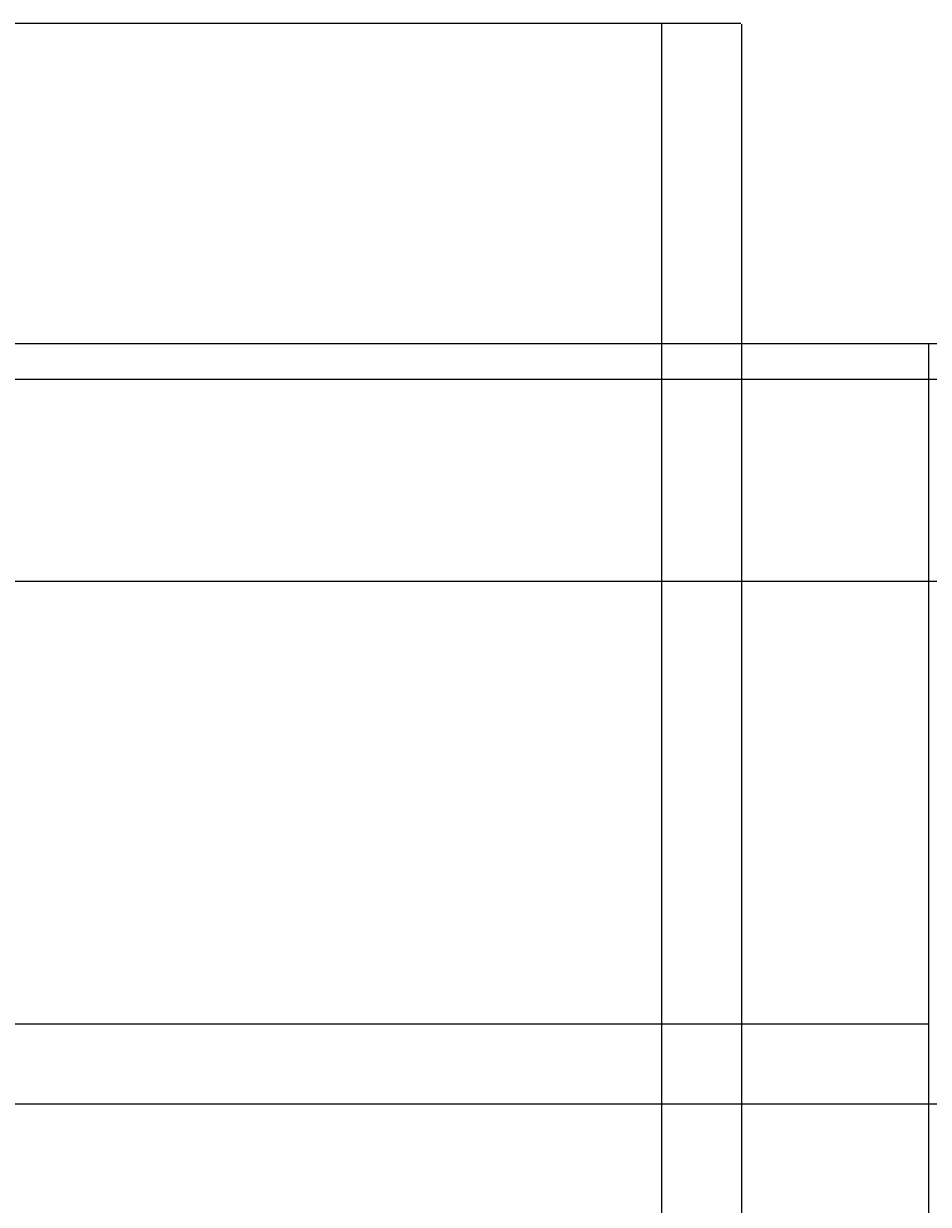
# Model space of a CAD drawing. Units: inches. Extents: x 867 to 1667, y -234 to 788.
# Tile 10 of 42: x 969 to 1071, y 125 to 258. Entities that reach past the tile are written whole.
import ezdxf

# ---------------------------------------------------------------- set-up
doc = ezdxf.new("R2010")
doc.units = ezdxf.units.IN
doc.header["$MEASUREMENT"] = 0
doc.layers.add('A-ANNO-DIMS', color=2, linetype='Continuous', lineweight=18)
doc.styles.get("Standard").update_dxf_attribs({"font": 'arial.ttf'})
doc.dimstyles.get("Standard").update_dxf_attribs({"dimtxt": 0.6875, "dimasz": 0.18, "dimexe": 0.18, "dimexo": 0.0625, "dimgap": 0.09, "dimtad": 0, "dimdec": 4, "dimzin": 0, "dimdsep": 46, "dimlunit": 4, "dimtxsty": 'Standard', "dimcen": 0.09, "dimadec": 0, "dimazin": 0, "dimtfac": 1, "dimtdec": 4, "dimtofl": 0, "dimtmove": 0, "dimatfit": 3, "dimfxl": 1, "dimtolj": 1, "dimtzin": 0, "dimarcsym": 0})

# ---------------------------------------------------------------- blocks, each defined once
blk = doc.blocks.new('*D37')
at = {"layer": 'A-ANNO-DIMS', "color": 0, "lineweight": -2, "transparency": 16777216}
for p, q in [((1049.89, 257.55), (1049.89, -233.54)), ((1196.89, 257.55), (1196.89, -233.54)), ((1050.07, -233.36), (1122.57, -233.36)), ((1196.71, -233.36), (1124.2, -233.36))]:
    blk.add_line(p, q, dxfattribs=at)
at = {"layer": 'A-ANNO-DIMS', "color": 0, "transparency": 16777216}
for points in [[(1050.07, -233.33), (1050.07, -233.39), (1049.89, -233.36)], [(1196.71, -233.33), (1196.71, -233.39), (1196.89, -233.36)]]:
    blk.add_solid(points, dxfattribs=at)
at = {"layer": 'Defpoints', "color": 0, "transparency": 16777216}
for p in [(1049.89, 257.62), (1196.89, 257.62), (1196.89, -233.36)]:
    blk.add_point(p, dxfattribs=at)
at = {"layer": 'A-ANNO-DIMS', "color": 0, "transparency": 16777216, "insert": (1123.39, -233.36), "char_height": 0.688, "attachment_point": 5}
blk.add_mtext('\\A1;147', dxfattribs=at)
blk = doc.blocks.new('*D39')
at = {"layer": 'A-ANNO-DIMS', "color": 0, "lineweight": -2, "transparency": 16777216}
for p, q in [((1040.82, 413.62), (867.76, 413.62)), ((867.94, 413.44), (867.94, 336.43)), ((867.94, 257.8), (867.94, 334.8)), ((1040.82, 257.62), (867.76, 257.62))]:
    blk.add_line(p, q, dxfattribs=at)
at = {"layer": 'A-ANNO-DIMS', "color": 0, "transparency": 16777216}
for points in [[(867.91, 413.44), (867.97, 413.44), (867.94, 413.62)], [(867.91, 257.8), (867.97, 257.8), (867.94, 257.62)]]:
    blk.add_solid(points, dxfattribs=at)
at = {"layer": 'Defpoints', "color": 0, "transparency": 16777216}
for p in [(867.94, 413.62), (1040.89, 413.62), (1040.89, 257.62)]:
    blk.add_point(p, dxfattribs=at)
at = {"layer": 'A-ANNO-DIMS', "color": 0, "transparency": 16777216, "insert": (867.94, 335.62), "char_height": 0.688, "attachment_point": 5, "rotation": 90}
blk.add_mtext('\\A1;156', dxfattribs=at)
blk = doc.blocks.new('*D40')
at = {"layer": 'A-ANNO-DIMS', "color": 0, "lineweight": -2, "transparency": 16777216}
for p, q in [((1040.82, 257.62), (867.76, 257.62)), ((867.94, 257.44), (867.94, 240.2)), ((867.94, 221.8), (867.94, 239.04)), ((1070.82, 221.62), (867.76, 221.62))]:
    blk.add_line(p, q, dxfattribs=at)
at = {"layer": 'A-ANNO-DIMS', "color": 0, "transparency": 16777216}
for points in [[(867.91, 257.44), (867.97, 257.44), (867.94, 257.62)], [(867.91, 221.8), (867.97, 221.8), (867.94, 221.62)]]:
    blk.add_solid(points, dxfattribs=at)
at = {"layer": 'Defpoints', "color": 0, "transparency": 16777216}
for p in [(1040.89, 257.62), (867.94, 221.62), (1070.89, 221.62)]:
    blk.add_point(p, dxfattribs=at)
at = {"layer": 'A-ANNO-DIMS', "color": 0, "transparency": 16777216, "insert": (867.94, 239.62), "char_height": 0.688, "attachment_point": 5, "rotation": 90}
blk.add_mtext('\\A1;36', dxfattribs=at)
blk = doc.blocks.new('*D41')
at = {"layer": 'A-ANNO-DIMS', "color": 0, "lineweight": -2, "transparency": 16777216}
for p, q in [((1149.82, 221.62), (867.76, 221.62)), ((867.94, 221.44), (867.94, 179.85)), ((867.94, 136.3), (867.94, 177.88)), ((1149.82, 136.12), (867.76, 136.12))]:
    blk.add_line(p, q, dxfattribs=at)
at = {"layer": 'A-ANNO-DIMS', "color": 0, "transparency": 16777216}
for points in [[(867.91, 221.44), (867.97, 221.44), (867.94, 221.62)], [(867.91, 136.3), (867.97, 136.3), (867.94, 136.12)]]:
    blk.add_solid(points, dxfattribs=at)
at = {"layer": 'Defpoints', "color": 0, "transparency": 16777216}
for p in [(867.94, 221.62), (1149.89, 221.62), (1149.89, 136.12)]:
    blk.add_point(p, dxfattribs=at)
at = {"layer": 'A-ANNO-DIMS', "color": 0, "transparency": 16777216, "insert": (867.94, 178.87), "char_height": 0.688, "attachment_point": 5, "rotation": 90}
blk.add_mtext('\\A1;85.5', dxfattribs=at)
blk = doc.blocks.new('*D44')
at = {"layer": 'A-ANNO-DIMS', "color": 0, "lineweight": -2, "transparency": 16777216}
for p, q in [((1070.82, 145.12), (867.76, 145.12)), ((867.94, 144.94), (867.94, 64.93)), ((867.94, -16.7), (867.94, 63.3)), ((1070.82, -16.88), (867.76, -16.88))]:
    blk.add_line(p, q, dxfattribs=at)
at = {"layer": 'A-ANNO-DIMS', "color": 0, "transparency": 16777216}
for points in [[(867.91, 144.94), (867.97, 144.94), (867.94, 145.12)], [(867.91, -16.7), (867.97, -16.7), (867.94, -16.88)]]:
    blk.add_solid(points, dxfattribs=at)
at = {"layer": 'Defpoints', "color": 0, "transparency": 16777216}
for p in [(867.94, 145.12), (1070.89, 145.12), (1070.89, -16.88)]:
    blk.add_point(p, dxfattribs=at)
at = {"layer": 'A-ANNO-DIMS', "color": 0, "transparency": 16777216, "insert": (867.94, 64.12), "char_height": 0.688, "attachment_point": 5, "rotation": 90}
blk.add_mtext('\\A1;162', dxfattribs=at)
blk = doc.blocks.new('*D56')
at = {"layer": 'A-ANNO-DIMS', "color": 0, "lineweight": -2, "transparency": 16777216}
for p, q in [((1049.82, 300.59), (867.76, 300.59)), ((867.94, 300.41), (867.94, 280.37)), ((867.94, 257.8), (867.94, 277.84)), ((1049.82, 257.62), (867.76, 257.62))]:
    blk.add_line(p, q, dxfattribs=at)
at = {"layer": 'A-ANNO-DIMS', "color": 0, "transparency": 16777216}
for points in [[(867.91, 300.41), (867.97, 300.41), (867.94, 300.59)], [(867.91, 257.8), (867.97, 257.8), (867.94, 257.62)]]:
    blk.add_solid(points, dxfattribs=at)
at = {"layer": 'Defpoints', "color": 0, "transparency": 16777216}
for p in [(867.94, 300.59), (1049.89, 300.59), (1049.89, 257.62)]:
    blk.add_point(p, dxfattribs=at)
at = {"layer": 'A-ANNO-DIMS', "color": 0, "transparency": 16777216, "insert": (867.94, 279.1), "char_height": 0.688, "attachment_point": 5, "rotation": 90}
blk.add_mtext('\\A1;42.97', dxfattribs=at)
blk = doc.blocks.new('*D61')
at = {"layer": 'A-ANNO-DIMS', "color": 0, "lineweight": -2, "transparency": 16777216}
for p, q in [((1076.39, 217.62), (867.76, 217.62)), ((867.94, 217.44), (867.94, 207.78)), ((867.94, 195.06), (867.94, 204.72)), ((1079.82, 194.88), (867.76, 194.88))]:
    blk.add_line(p, q, dxfattribs=at)
at = {"layer": 'A-ANNO-DIMS', "color": 0, "transparency": 16777216}
for points in [[(867.91, 217.44), (867.97, 217.44), (867.94, 217.62)], [(867.91, 195.06), (867.97, 195.06), (867.94, 194.88)]]:
    blk.add_solid(points, dxfattribs=at)
at = {"layer": 'Defpoints', "color": 0, "transparency": 16777216}
for p in [(867.94, 217.62), (1076.46, 217.62), (1079.89, 194.88)]:
    blk.add_point(p, dxfattribs=at)
at = {"layer": 'A-ANNO-DIMS', "color": 0, "transparency": 16777216, "insert": (867.94, 206.25), "char_height": 0.688, "attachment_point": 5, "rotation": 90}
blk.add_mtext('\\A1;22.735', dxfattribs=at)
blk = doc.blocks.new('*D63')
at = {"layer": 'A-ANNO-DIMS', "color": 0, "lineweight": -2, "transparency": 16777216}
for p, q in [((1040.89, 257.55), (1040.89, -233.54)), ((1070.89, 221.55), (1070.89, -233.54)), ((1041.07, -233.36), (1055.31, -233.36)), ((1070.71, -233.36), (1056.47, -233.36))]:
    blk.add_line(p, q, dxfattribs=at)
at = {"layer": 'A-ANNO-DIMS', "color": 0, "transparency": 16777216}
for points in [[(1041.07, -233.33), (1041.07, -233.39), (1040.89, -233.36)], [(1070.71, -233.33), (1070.71, -233.39), (1070.89, -233.36)]]:
    blk.add_solid(points, dxfattribs=at)
at = {"layer": 'Defpoints', "color": 0, "transparency": 16777216}
for p in [(1040.89, 257.62), (1070.89, 221.62), (1070.89, -233.36)]:
    blk.add_point(p, dxfattribs=at)
at = {"layer": 'A-ANNO-DIMS', "color": 0, "transparency": 16777216, "insert": (1055.89, -233.36), "char_height": 0.688, "attachment_point": 5}
blk.add_mtext('\\A1;30', dxfattribs=at)

msp = doc.modelspace()

# ---------------------------------------------------------------- dimensions: what is measured, and where the dimension line sits
at = {"layer": 'A-ANNO-DIMS'}
for base, p1, p2, override, picture, middle in [((867.9366, 413.617), (1040.8866, 257.617), (1040.8866, 413.617), {"dimdec": 0, "dimlfac": 1, "dimrnd": 0, "dimzin": 0, "dimdsep": 46, "dimlunit": 2}, '*D39', (867.9366, 335.617)), ((867.9366, 300.5856), (1049.8866, 257.617), (1049.8866, 300.5856), {"dimdec": 2, "dimlfac": 1, "dimrnd": 0, "dimzin": 0, "dimdsep": 46, "dimlunit": 2}, '*D56', (867.9366, 279.1013)), ((867.9366, 221.617), (1040.8866, 257.617), (1070.8866, 221.617), {"dimdec": 0, "dimlfac": 1, "dimrnd": 0, "dimzin": 0, "dimdsep": 46, "dimlunit": 2}, '*D40', (867.9366, 239.617)), ((867.9366, 221.617), (1149.8866, 136.117), (1149.8866, 221.617), {"dimdec": 1, "dimlfac": 1, "dimrnd": 0, "dimzin": 0, "dimdsep": 46, "dimlunit": 2}, '*D41', (867.9366, 178.867)), ((867.9366, 217.617), (1079.8866, 194.8824), (1076.4575, 217.617), {"dimdec": 3, "dimlfac": 1, "dimrnd": 0, "dimzin": 0, "dimdsep": 46, "dimlunit": 2}, '*D61', (867.9366, 206.2497)), ((867.9366, 145.117), (1070.8866, -16.883), (1070.8866, 145.117), {"dimdec": 0, "dimlfac": 1, "dimrnd": 0, "dimzin": 0, "dimdsep": 46, "dimlunit": 2}, '*D44', (867.9366, 64.117))]:
    dim = msp.add_linear_dim(base=base, p1=p1, p2=p2, angle=90, dimstyle='Standard', override=override, dxfattribs=at)
    dim.commit()
    dim.dimension.update_dxf_attribs({"geometry": picture, "text_midpoint": middle})
for base, p1, p2, picture, middle in [((1070.8866, -233.3581), (1040.8866, 257.617), (1070.8866, 221.617), '*D63', (1055.8866, -233.3581)), ((1196.8866, -233.3581), (1049.8866, 257.617), (1196.8866, 257.617), '*D37', (1123.3866, -233.3581))]:
    dim = msp.add_linear_dim(base=base, p1=p1, p2=p2, dimstyle='Standard', override={"dimdec": 0, "dimlfac": 1, "dimrnd": 0, "dimzin": 0, "dimdsep": 46, "dimlunit": 2}, dxfattribs=at)
    dim.commit()
    dim.dimension.update_dxf_attribs({"geometry": picture, "text_midpoint": middle})

doc.saveas('drawing.dxf')
